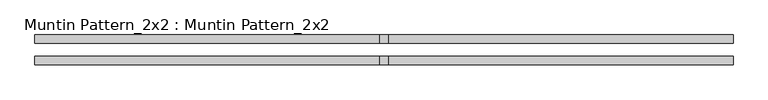
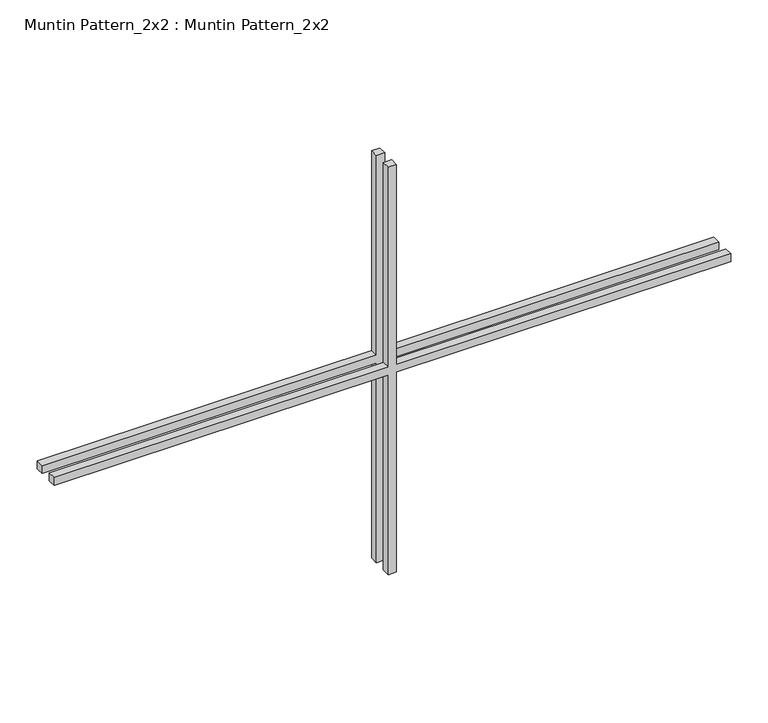
"""IFC4 building model written with IfcOpenShell, lengths in millimetres: proxy geometry, Muntin Pattern_2x2 : Muntin Pattern_2x2."""

from ifc_helpers import new_model, si_unit, frame, origin, place, context, project, spatial, polyline, outline, extrude, source, transform, mapped, element, save


def muntin_pattern_2x2_muntin_pattern_2x2_872d1288(model_context):
    return source(origin(), model_context, "Body", "SweptSolid", [
        extrude(outline(polyline([(338.1375, -6.35), (338.1375, -520.7), (325.4375, -520.7), (325.4375, -6.35), (0.0, -6.35), (0.0, 6.35), (325.4375, 6.35), (325.4375, 520.7), (338.1375, 520.7), (338.1375, 6.35), (663.575, 6.35), (663.575, -6.35), (338.1375, -6.35)])), frame((0.0, 9.525, 0.0), z_axis=(0.0, 1.0, 0.0), x_axis=(0.0, 0.0, 1.0)), (0.0, 0.0, 1.0), 12.7),
        extrude(outline(polyline([(338.1375, -6.35), (338.1375, -520.7), (325.4375, -520.7), (325.4375, -6.35), (0.0, -6.35), (0.0, 6.35), (325.4375, 6.35), (325.4375, 520.7), (338.1375, 520.7), (338.1375, 6.35), (663.575, 6.35), (663.575, -6.35), (338.1375, -6.35)])), frame((0.0, -22.225, 0.0), z_axis=(0.0, 1.0, 0.0), x_axis=(0.0, 0.0, 1.0)), (0.0, 0.0, 1.0), 12.7),
    ])


if __name__ == "__main__":
    model = new_model("IFC4")
    model_context = context("Model", 3, world=origin())
    ifc_project = project(units=[si_unit("LENGTHUNIT", "METRE", prefix="MILLI")], contexts=[model_context])
    site = spatial("IfcSite", under=ifc_project)
    building = spatial("IfcBuilding", under=site)
    placement = place(None, origin())
    muntin_pattern_2x2_muntin_pattern_2x2_shape = muntin_pattern_2x2_muntin_pattern_2x2_872d1288(model_context)
    element("IfcBuildingElementProxy", 1, Name="Muntin Pattern_2x2 : Muntin Pattern_2x2", ObjectType="Muntin Pattern_2x2 : Muntin Pattern_2x2", at=placement, inside=building, context=model_context, shape_type="MappedRepresentation", body=[
        mapped(muntin_pattern_2x2_muntin_pattern_2x2_shape, transform((0.0, 0.0, 0.0), x_axis=(1.0, 0.0, 0.0), y_axis=(0.0, 1.0, 0.0), z_axis=(0.0, 0.0, 1.0))),
    ])
    save(model, "model.ifc")

# Revit data of these elements
# Type "Muntin Pattern_2x2 : Muntin Pattern_2x2"
#   Width [instance default] = 4' - 0"
#   Thickness = 0' - 0 1/2"
#   Height [instance default] = 4' - 0"
#   Distance = 0' - 0 3/4"
#   Interior Material [instance default] = none
#   Exterior Material [instance default] = none
#   Default Elevation = 0
# Element 1 (IfcBuildingElementProxy, "Muntin Pattern_2x2 : Muntin Pattern_2x2")
#   Width = 3' - 5"
#   Height = 2' - 2 1/8"
#   Interior Material = Wood - Stained
#   Exterior Material = Clad - White
#   Materials on its faces: "Clad - White", "Wood - Stained"
# Materials
#   "Clad - White": class "Wood", colour RGB 242 242 238, transparency 0, Cost = 0
#   "Wood - Stained": class "Wood", colour RGB 224 178 126, transparency 0, Cost = 0
